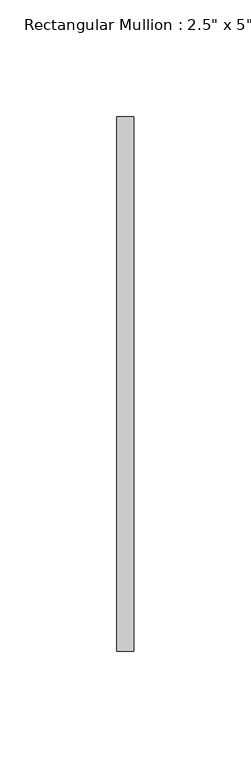
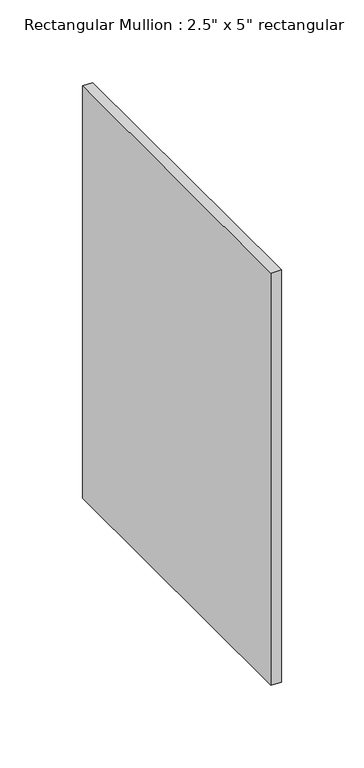
"""IFC4 building model written with IfcOpenShell, lengths in millimetres: member geometry."""

from ifc_helpers import new_model, si_unit, frame, origin, place, context, project, spatial, polyline, outline, extrude, source, transform, mapped, element, save


def member_b53b5e8d(model_context):
    return source(origin(), model_context, "Body", "SweptSolid", [
        extrude(outline(polyline([(3.6195, 114.3), (3.6195, -114.3), (-3.6195, -114.3), (-3.6195, 114.3), (3.6195, 114.3)])), frame((0.0, 0.0, -304.8), z_axis=(0.0, 0.0, 1.0), x_axis=(1.0, 0.0, 0.0)), (0.0, 0.0, 1.0), 304.8),
    ])


if __name__ == "__main__":
    model = new_model("IFC4")
    model_context = context("Model", 3, world=origin())
    ifc_project = project(units=[si_unit("LENGTHUNIT", "METRE", prefix="MILLI")], contexts=[model_context])
    site = spatial("IfcSite", under=ifc_project)
    building = spatial("IfcBuilding", under=site)
    placement = place(None, origin())
    member_shape = member_b53b5e8d(model_context)
    element("IfcMember", 1, ObjectType="Rectangular Mullion : 2.5\" x 5\" rectangular", at=placement, inside=building, context=model_context, shape_type="MappedRepresentation", body=[
        mapped(member_shape, transform((0.0, 0.0, 0.0), x_axis=(1.0, 0.0, 0.0), y_axis=(0.0, 1.0, 0.0), z_axis=(0.0, 0.0, 1.0))),
    ])
    save(model, "model.ifc")

# Revit data of these elements
# Type "Rectangular Mullion : 2.5\" x 5\" rectangular"
#   built-in parameter 1007304 = 0.75 (stored number, unit not read)
#   built-in parameter 1007301 = 0.011875 (stored number, unit not read)
#   built-in parameter 1007300 = 0.011875 (stored number, unit not read)
# Element 1 (IfcMember, "Rectangular Mullion : 2.5\" x 5\" rectangular")
#   Materials on its faces: "WINDOW GLASS MATERIAL"
# Materials
#   "WINDOW GLASS MATERIAL": class "Generic", colour RGB 120 120 120, transparency 0, Cost = 0
